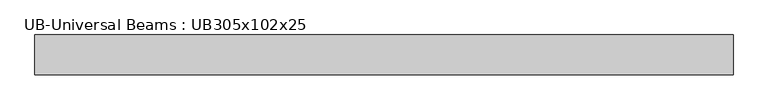
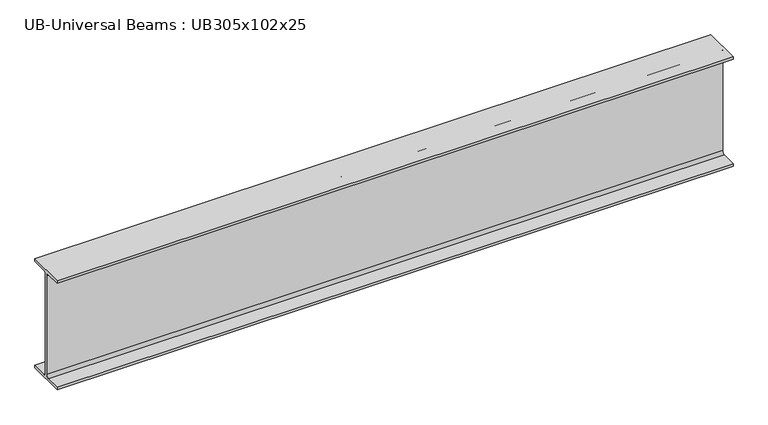
"""IFC4 building model written with IfcOpenShell, lengths in millimetres: beam geometry, UB-Universal Beams : UB305x102x25."""

from ifc_helpers import new_model, si_unit, point, frame, frame_2d, origin, place, context, project, spatial, polyline, circle_curve, trimmed, segment, composite_curve, outline, extrude, source, transform, mapped, element, save


def ub_universal_beams_ub305x102x25_1ce1eee3(model_context):
    return source(origin(), model_context, "Body", "SweptSolid", [
        extrude(outline(composite_curve([segment(polyline([(50.8, -145.55), (50.8, -152.55), (-50.8, -152.55), (-50.8, -145.55), (-10.5, -145.55)]), True, "CONTINUOUS"), segment(trimmed(circle_curve(frame_2d((-10.5, -137.95)), 7.6), [point((-10.5, -145.55))], [point((-2.9, -137.95))], True, "CARTESIAN"), True, "CONTINUOUS"), segment(polyline([(-2.9, -137.95), (-2.9, 137.95)]), True, "CONTINUOUS"), segment(trimmed(circle_curve(frame_2d((-10.5, 137.95)), 7.6), [point((-2.9, 137.95))], [point((-10.5, 145.55))], True, "CARTESIAN"), True, "CONTINUOUS"), segment(polyline([(-10.5, 145.55), (-50.8, 145.55), (-50.8, 152.55), (50.8, 152.55), (50.8, 145.55), (10.5, 145.55)]), True, "CONTINUOUS"), segment(trimmed(circle_curve(frame_2d((10.5, 137.95)), 7.6), [point((10.5, 145.55))], [point((2.9, 137.95))], True, "CARTESIAN"), True, "CONTINUOUS"), segment(polyline([(2.9, 137.95), (2.9, -137.95)]), True, "CONTINUOUS"), segment(trimmed(circle_curve(frame_2d((10.5, -137.95)), 7.6), [point((2.9, -137.95))], [point((10.5, -145.55))], True, "CARTESIAN"), True, "CONTINUOUS"), segment(polyline([(10.5, -145.55), (50.8, -145.55)]), True, "CONTINUOUS")], self_intersect=False)), frame((-757.55, 0.0, 0.0), z_axis=(1.0, 0.0, 0.0), x_axis=(0.0, 1.0, 0.0)), (0.0, 0.0, 1.0), 1787.1),
    ])


if __name__ == "__main__":
    model = new_model("IFC4")
    model_context = context("Model", 3, world=origin())
    ifc_project = project(units=[si_unit("LENGTHUNIT", "METRE", prefix="MILLI")], contexts=[model_context])
    site = spatial("IfcSite", under=ifc_project)
    building = spatial("IfcBuilding", under=site)
    placement = place(None, origin())
    ub_universal_beams_ub305x102x25_shape = ub_universal_beams_ub305x102x25_1ce1eee3(model_context)
    element("IfcBeam", 1, ObjectType="UB-Universal Beams : UB305x102x25", at=placement, inside=building, context=model_context, shape_type="MappedRepresentation", body=[
        mapped(ub_universal_beams_ub305x102x25_shape, transform((0.0, 0.0, 0.0), x_axis=(1.0, 0.0, 0.0), y_axis=(0.0, 1.0, 0.0), z_axis=(0.0, 0.0, 1.0))),
    ])
    save(model, "model.ifc")

# Revit data of these elements
# Type "UB-Universal Beams : UB305x102x25"
#   Section Name Key = "UB305X102X25"
#   Width = 10.16 cm
#   Web Thickness = 0.58 cm
#   Web Fillet = 0.76 cm
#   Warping Constant = 27300.0 cm⁶
#   Torsional Moment of Inertia = 4.77 cm⁴
#   Section Area = 31.6 cm²
#   Plastic Modulus weak axis = 39.0 cm³
#   Plastic Modulus strong axis = 342.0 cm³
#   Nominal Weight = 24.7999 kgf/m
#   Moment of Inertia weak axis = 123.00 cm⁴
#   Moment of Inertia strong axis = 4455.00 cm⁴
#   Height = 30.51 cm
#   Flange Thickness = 0.7 cm
#   Elastic Modulus weak axis = 24.2 cm³
#   Elastic Modulus strong axis = 292.0 cm³
#   Centroid Vertical = 15.255 cm
#   Centroid Horizontal = 5.08 cm
#   Bolt Spacing = 5.4 cm
#   Length [instance default] = 1.5 m
#   Structural Material [instance default] = Metal - Steel 43-275
#   Type Comments = ""
#   Assembly Code = ""
# Element 1 (IfcBeam, "UB-Universal Beams : UB305x102x25")
#   Materials on its faces: "Metal - Steel 43-275"
# Materials
#   "Metal - Steel 43-275": class "Metal", colour RGB 247 247 247, transparency 0, Cost = 0
